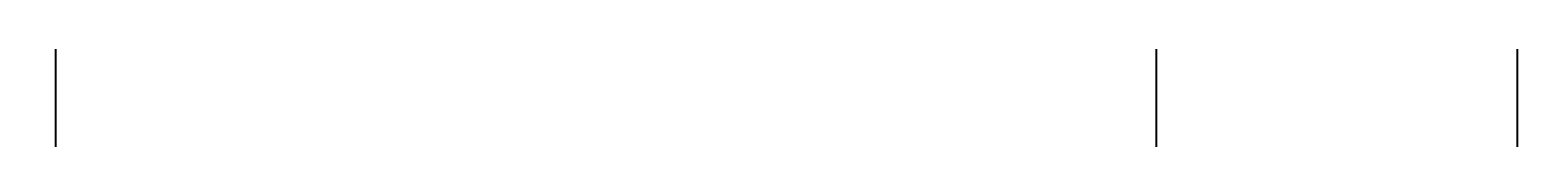
# Model space of a CAD drawing. Units: inches. Extents: x 35362 to 73946, y 43607 to 67532.
# Tile 83 of 134: x 50119 to 51337, y 47625 to 47689. Entities that reach past the tile are written whole.
import ezdxf

# ---------------------------------------------------------------- set-up
doc = ezdxf.new("R2010")
doc.units = ezdxf.units.IN
doc.header["$MEASUREMENT"] = 0
doc.layers.add('A-ANNO-DIMS', color=2, linetype='Continuous', lineweight=18)
doc.styles.get("Standard").update_dxf_attribs({"font": 'arial.ttf'})
doc.dimstyles.get("Standard").update_dxf_attribs({"dimtxt": 0.18, "dimasz": 0.18, "dimexe": 0.18, "dimexo": 0.0625, "dimgap": 0.09, "dimtad": 0, "dimtih": 1, "dimtoh": 1, "dimdec": 4, "dimzin": 0, "dimdsep": 46, "dimtxsty": 'Standard', "dimcen": 0.09, "dimadec": 0, "dimazin": 0, "dimtfac": 1, "dimtdec": 4, "dimtofl": 0, "dimtmove": 0, "dimatfit": 3, "dimfxl": 1, "dimtolj": 1, "dimtzin": 0, "dimarcsym": 0})

# ---------------------------------------------------------------- blocks, each defined once
blk = doc.blocks.new('*D11')
at = {"layer": 'A-ANNO-DIMS', "color": 0, "lineweight": -2, "transparency": 16777216}
for p, q in [((47978.7, 56028.8), (47978.7, 43606.7)), ((53109.8, 56028.8), (53109.8, 43606.7)), ((47978.8, 43606.9), (50543.9, 43606.9)), ((53109.6, 43606.9), (50544.6, 43606.9))]:
    blk.add_line(p, q, dxfattribs=at)
at = {"layer": 'A-ANNO-DIMS', "color": 0, "transparency": 16777216}
for points in [[(47978.8, 43606.9), (47978.8, 43606.8), (47978.7, 43606.9)], [(53109.6, 43606.9), (53109.6, 43606.8), (53109.8, 43606.9)]]:
    blk.add_solid(points, dxfattribs=at)
at = {"layer": 'Defpoints', "color": 0, "transparency": 16777216}
for p in [(47978.7, 56028.8), (53109.8, 56028.8), (53109.8, 43606.9)]:
    blk.add_point(p, dxfattribs=at)
at = {"layer": 'A-ANNO-DIMS', "color": 0, "transparency": 16777216, "insert": (50544.2, 43606.9), "char_height": 0.18, "attachment_point": 5}
blk.add_mtext('\\A1;5131', dxfattribs=at)
blk = doc.blocks.new('*D13')
at = {"layer": 'A-ANNO-DIMS', "color": 0, "lineweight": -2, "transparency": 16777216}
for p, q in [((48373.5, 51694), (48373.5, 43606.7)), ((51029, 51694), (51029, 43606.7)), ((48373.7, 43606.9), (49700.8, 43606.9)), ((51028.9, 43606.9), (49701.7, 43606.9))]:
    blk.add_line(p, q, dxfattribs=at)
at = {"layer": 'A-ANNO-DIMS', "color": 0, "transparency": 16777216}
for points in [[(48373.7, 43606.9), (48373.7, 43606.8), (48373.5, 43606.9)], [(51028.9, 43606.9), (51028.9, 43606.8), (51029, 43606.9)]]:
    blk.add_solid(points, dxfattribs=at)
at = {"layer": 'Defpoints', "color": 0, "transparency": 16777216}
for p in [(48373.5, 51694.1), (51029, 51694.1), (51029, 43606.9)]:
    blk.add_point(p, dxfattribs=at)
at = {"layer": 'A-ANNO-DIMS', "color": 0, "transparency": 16777216, "insert": (49701.3, 43606.9), "char_height": 0.18, "attachment_point": 5}
blk.add_mtext('\\A1;2655.6', dxfattribs=at)
blk = doc.blocks.new('*D17')
at = {"layer": 'A-ANNO-DIMS', "color": 0, "lineweight": -2, "transparency": 16777216}
for p, q in [((49923.3, 61293.2), (49923.3, 43606.7)), ((51913.9, 61293.2), (51913.9, 43606.7)), ((49923.5, 43606.9), (50918.2, 43606.9)), ((51913.8, 43606.9), (50919.1, 43606.9))]:
    blk.add_line(p, q, dxfattribs=at)
at = {"layer": 'A-ANNO-DIMS', "color": 0, "transparency": 16777216}
for points in [[(49923.5, 43606.9), (49923.5, 43606.8), (49923.3, 43606.9)], [(51913.8, 43606.9), (51913.8, 43606.8), (51913.9, 43606.9)]]:
    blk.add_solid(points, dxfattribs=at)
at = {"layer": 'Defpoints', "color": 0, "transparency": 16777216}
for p in [(49923.3, 61293.3), (51913.9, 61293.3), (51913.9, 43606.9)]:
    blk.add_point(p, dxfattribs=at)
at = {"layer": 'A-ANNO-DIMS', "color": 0, "transparency": 16777216, "insert": (50918.6, 43606.9), "char_height": 0.18, "attachment_point": 5}
blk.add_mtext('\\A1;1990.6', dxfattribs=at)
blk = doc.blocks.new('*D67')
at = {"layer": 'A-ANNO-DIMS', "color": 0, "lineweight": -2, "transparency": 16777216}
for p, q in [((56873.5, 53351.5), (35361.8, 53351.5)), ((35361.9, 53351.3), (35361.9, 49400.9)), ((35361.9, 45450.1), (35361.9, 49400.5)), ((53793.6, 45449.9), (35361.8, 45449.9))]:
    blk.add_line(p, q, dxfattribs=at)
at = {"layer": 'A-ANNO-DIMS', "color": 0, "transparency": 16777216}
for points in [[(35361.9, 53351.3), (35362, 53351.3), (35361.9, 53351.5)], [(35361.9, 45450.1), (35362, 45450.1), (35361.9, 45449.9)]]:
    blk.add_solid(points, dxfattribs=at)
at = {"layer": 'Defpoints', "color": 0, "transparency": 16777216}
for p in [(35361.9, 53351.5), (56873.6, 53351.5), (53793.6, 45449.9)]:
    blk.add_point(p, dxfattribs=at)
at = {"layer": 'A-ANNO-DIMS', "color": 0, "transparency": 16777216, "insert": (35361.9, 49400.7), "char_height": 0.18, "attachment_point": 5}
blk.add_mtext('\\A1;7901.6', dxfattribs=at)
blk = doc.blocks.new('*D87')
at = {"layer": 'A-ANNO-DIMS', "color": 0, "lineweight": -2, "transparency": 16777216}
for p, q in [((52362.5, 48318.3), (35361.8, 48318.3)), ((35361.9, 48318.1), (35361.9, 47931.4)), ((35361.9, 47544.3), (35361.9, 47931)), ((52362.5, 47544.1), (35361.8, 47544.1))]:
    blk.add_line(p, q, dxfattribs=at)
at = {"layer": 'A-ANNO-DIMS', "color": 0, "transparency": 16777216}
for points in [[(35361.9, 48318.1), (35362, 48318.1), (35361.9, 48318.3)], [(35361.9, 47544.3), (35362, 47544.3), (35361.9, 47544.1)]]:
    blk.add_solid(points, dxfattribs=at)
at = {"layer": 'Defpoints', "color": 0, "transparency": 16777216}
for p in [(35361.9, 48318.3), (52362.6, 48318.3), (52362.6, 47544.1)]:
    blk.add_point(p, dxfattribs=at)
at = {"layer": 'A-ANNO-DIMS', "color": 0, "transparency": 16777216, "insert": (35361.9, 47931.2), "char_height": 0.18, "attachment_point": 5}
blk.add_mtext('\\A1;774.1', dxfattribs=at)
blk = doc.blocks.new('*D107')
at = {"layer": 'A-ANNO-DIMS', "color": 0, "lineweight": -2, "transparency": 16777216}
for p, q in [((50139.6, 59850), (50139.6, 43606.7)), ((51320.8, 59850), (51320.8, 43606.7)), ((50139.7, 43606.9), (50729.7, 43606.9)), ((51320.6, 43606.9), (50730.6, 43606.9))]:
    blk.add_line(p, q, dxfattribs=at)
at = {"layer": 'A-ANNO-DIMS', "color": 0, "transparency": 16777216}
for points in [[(50139.7, 43606.9), (50139.7, 43606.8), (50139.6, 43606.9)], [(51320.6, 43606.9), (51320.6, 43606.8), (51320.8, 43606.9)]]:
    blk.add_solid(points, dxfattribs=at)
at = {"layer": 'Defpoints', "color": 0, "transparency": 16777216}
for p in [(50139.6, 59850.1), (51320.8, 59850.1), (51320.8, 43606.9)]:
    blk.add_point(p, dxfattribs=at)
at = {"layer": 'A-ANNO-DIMS', "color": 0, "transparency": 16777216, "insert": (50730.2, 43606.9), "char_height": 0.18, "attachment_point": 5}
blk.add_mtext('\\A1;1181.3', dxfattribs=at)

msp = doc.modelspace()

# ---------------------------------------------------------------- dimensions: what is measured, and where the dimension line sits
at = {"layer": 'A-ANNO-DIMS'}
for base, p1, p2, override, picture, middle in [((51913.931, 43606.859), (49923.307, 61293.286), (51913.931, 61293.286), {"dimdec": 1, "dimlfac": 1, "dimrnd": 0, "dimzin": 0, "dimdsep": 46, "dimlunit": 2}, '*D17', (50918.619, 43606.859)), ((51320.8133, 43606.859), (50139.5627, 59850.0769), (51320.8133, 59850.0769), {"dimdec": 1, "dimlfac": 1, "dimrnd": 0, "dimzin": 0, "dimdsep": 46, "dimlunit": 2}, '*D107', (50730.188, 43606.859)), ((53109.76, 43606.859), (47978.665, 56028.836), (53109.76, 56028.836), {"dimdec": 0, "dimlfac": 1, "dimrnd": 0, "dimzin": 0, "dimdsep": 46, "dimlunit": 2}, '*D11', (50544.212, 43606.859)), ((51029.043, 43606.859), (48373.492, 51694.087), (51029.043, 51694.087), {"dimdec": 1, "dimlfac": 1, "dimrnd": 0, "dimzin": 0, "dimdsep": 46, "dimlunit": 2}, '*D13', (49701.267, 43606.859))]:
    dim = msp.add_linear_dim(base=base, p1=p1, p2=p2, dimstyle='Standard', override=override, dxfattribs=at)
    dim.commit()
    dim.dimension.update_dxf_attribs({"geometry": picture, "text_midpoint": middle})
for base, p1, p2, picture, middle in [((35361.949, 53351.529), (53793.638, 45449.894), (56873.602, 53351.529), '*D67', (35361.949, 49400.712)), ((35361.949, 48318.269), (52362.557, 47544.134), (52362.557, 48318.269), '*D87', (35361.949, 47931.201))]:
    dim = msp.add_linear_dim(base=base, p1=p1, p2=p2, angle=90, dimstyle='Standard', override={"dimdec": 1, "dimlfac": 1, "dimrnd": 0, "dimzin": 0, "dimdsep": 46, "dimlunit": 2}, dxfattribs=at)
    dim.commit()
    dim.dimension.update_dxf_attribs({"geometry": picture, "text_midpoint": middle})

doc.saveas('drawing.dxf')
